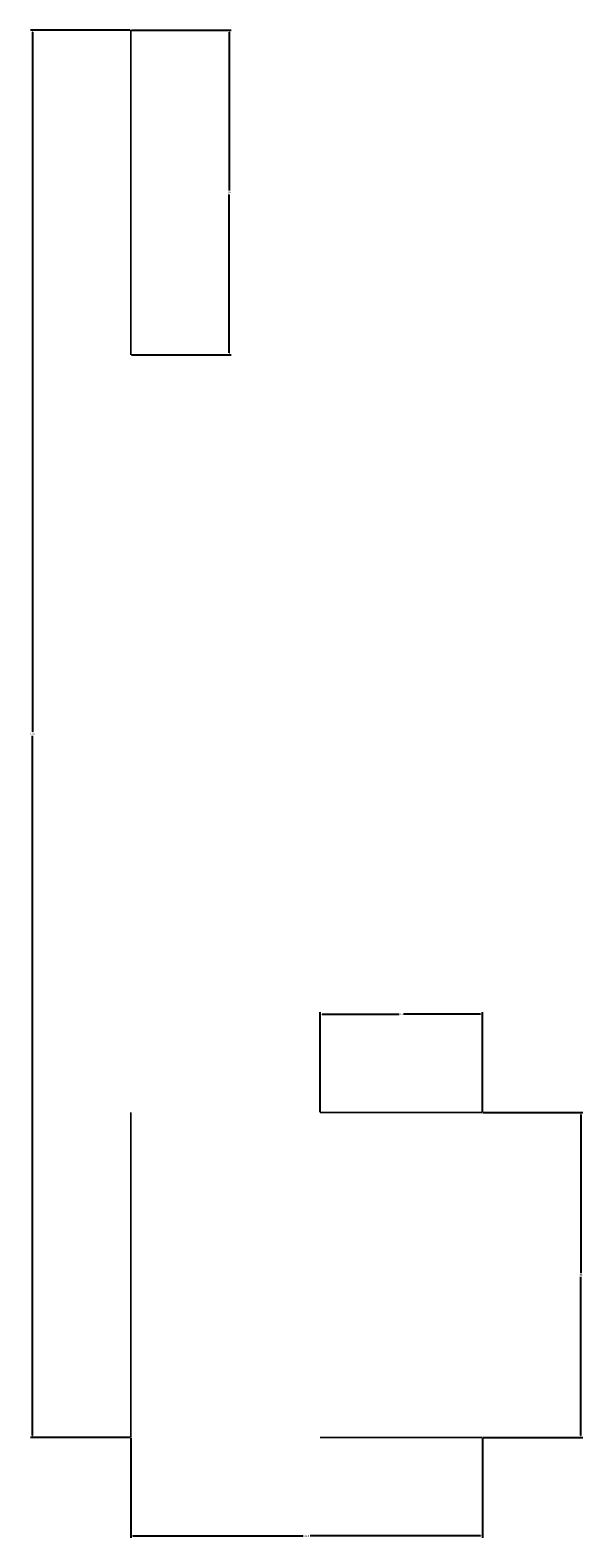
# Model space of a CAD drawing. Units: millimetres. Extents: x -9 to 42, y 320 to 460.
import ezdxf

# ---------------------------------------------------------------- set-up
doc = ezdxf.new("R2010")
doc.units = ezdxf.units.MM
doc.layers.add('M-CONS', color=8, linetype='Continuous', lineweight=13)
doc.layers.add('M-DIMS', color=2, linetype='Continuous', lineweight=18)
doc.styles.get("Standard").update_dxf_attribs({"font": 'arial.ttf'})
doc.dimstyles.get("Standard").update_dxf_attribs({"dimtxt": 0.18, "dimasz": 0.18, "dimexe": 0.18, "dimexo": 0.0625, "dimgap": 0.09, "dimtad": 0, "dimtih": 1, "dimtoh": 1, "dimdec": 4, "dimzin": 0, "dimdsep": 46, "dimtxsty": 'Standard', "dimcen": 0.09, "dimadec": 0, "dimazin": 0, "dimtfac": 1, "dimtdec": 4, "dimtofl": 0, "dimtmove": 0, "dimatfit": 3, "dimfxl": 1, "dimtolj": 1, "dimtzin": 0, "dimarcsym": 0})

# ---------------------------------------------------------------- blocks, each defined once
blk = doc.blocks.new('*D3')
at = {"layer": 'Defpoints', "color": 0, "transparency": 16777216}
for p in [(0, 329.55), (32.5, 329.55), (32.5, 320.45)]:
    blk.add_point(p, dxfattribs=at)
at = {"layer": 'M-DIMS', "color": 0, "lineweight": -2, "transparency": 16777216}
for p, q in [((0, 329.49), (0, 320.27)), ((32.5, 329.49), (32.5, 320.27)), ((0.18, 320.45), (15.93, 320.45)), ((32.32, 320.45), (16.57, 320.45))]:
    blk.add_line(p, q, dxfattribs=at)
at = {"layer": 'M-DIMS', "color": 0, "transparency": 16777216}
for points in [[(0.18, 320.48), (0.18, 320.42), (0, 320.45)], [(32.32, 320.48), (32.32, 320.42), (32.5, 320.45)]]:
    blk.add_solid(points, dxfattribs=at)
at = {"layer": 'M-DIMS', "color": 0, "transparency": 16777216, "insert": (16.25, 320.45), "char_height": 0.18, "attachment_point": 5}
blk.add_mtext('\\A1;32.5', dxfattribs=at)
blk = doc.blocks.new('*D4')
at = {"layer": 'Defpoints', "color": 0, "transparency": 16777216}
for p in [(32.5, 368.65), (17.5, 359.55), (32.5, 359.55)]:
    blk.add_point(p, dxfattribs=at)
at = {"layer": 'M-DIMS', "color": 0, "lineweight": -2, "transparency": 16777216}
for p, q in [((17.5, 359.61), (17.5, 368.83)), ((17.68, 368.65), (24.79, 368.65)), ((32.32, 368.65), (25.21, 368.65)), ((32.5, 359.61), (32.5, 368.83))]:
    blk.add_line(p, q, dxfattribs=at)
at = {"layer": 'M-DIMS', "color": 0, "transparency": 16777216}
for points in [[(17.68, 368.68), (17.68, 368.62), (17.5, 368.65)], [(32.32, 368.68), (32.32, 368.62), (32.5, 368.65)]]:
    blk.add_solid(points, dxfattribs=at)
at = {"layer": 'M-DIMS', "color": 0, "transparency": 16777216, "insert": (25, 368.65), "char_height": 0.18, "attachment_point": 5}
blk.add_mtext('\\A1;15', dxfattribs=at)
blk = doc.blocks.new('*D5')
at = {"layer": 'Defpoints', "color": 0, "transparency": 16777216}
for p in [(-9.1, 459.55), (0, 459.55), (0, 329.55)]:
    blk.add_point(p, dxfattribs=at)
at = {"layer": 'M-DIMS', "color": 0, "lineweight": -2, "transparency": 16777216}
for p, q in [((-0.06, 459.55), (-9.28, 459.55)), ((-9.1, 459.37), (-9.1, 394.73)), ((-9.1, 329.73), (-9.1, 394.37)), ((-0.06, 329.55), (-9.28, 329.55))]:
    blk.add_line(p, q, dxfattribs=at)
at = {"layer": 'M-DIMS', "color": 0, "transparency": 16777216}
for points in [[(-9.13, 459.37), (-9.07, 459.37), (-9.1, 459.55)], [(-9.13, 329.73), (-9.07, 329.73), (-9.1, 329.55)]]:
    blk.add_solid(points, dxfattribs=at)
at = {"layer": 'M-DIMS', "color": 0, "transparency": 16777216, "insert": (-9.1, 394.55), "char_height": 0.18, "attachment_point": 5}
blk.add_mtext('\\A1;130', dxfattribs=at)
blk = doc.blocks.new('*D6')
at = {"layer": 'Defpoints', "color": 0, "transparency": 16777216}
for p in [(0, 459.55), (0, 429.55), (9.1, 429.55)]:
    blk.add_point(p, dxfattribs=at)
at = {"layer": 'M-DIMS', "color": 0, "lineweight": -2, "transparency": 16777216}
for p, q in [((0.06, 459.55), (9.28, 459.55)), ((9.1, 459.37), (9.1, 444.73)), ((9.1, 429.73), (9.1, 444.37)), ((0.06, 429.55), (9.28, 429.55))]:
    blk.add_line(p, q, dxfattribs=at)
at = {"layer": 'M-DIMS', "color": 0, "transparency": 16777216}
for points in [[(9.07, 459.37), (9.13, 459.37), (9.1, 459.55)], [(9.07, 429.73), (9.13, 429.73), (9.1, 429.55)]]:
    blk.add_solid(points, dxfattribs=at)
at = {"layer": 'M-DIMS', "color": 0, "transparency": 16777216, "insert": (9.1, 444.55), "char_height": 0.18, "attachment_point": 5}
blk.add_mtext('\\A1;30', dxfattribs=at)
blk = doc.blocks.new('*D7')
at = {"layer": 'Defpoints', "color": 0, "transparency": 16777216}
for p in [(32.5, 359.55), (41.6, 359.55), (32.5, 329.55)]:
    blk.add_point(p, dxfattribs=at)
at = {"layer": 'M-DIMS', "color": 0, "lineweight": -2, "transparency": 16777216}
for p, q in [((32.56, 359.55), (41.78, 359.55)), ((41.6, 359.37), (41.6, 344.73)), ((41.6, 329.73), (41.6, 344.37)), ((32.56, 329.55), (41.78, 329.55))]:
    blk.add_line(p, q, dxfattribs=at)
at = {"layer": 'M-DIMS', "color": 0, "transparency": 16777216}
for points in [[(41.57, 359.37), (41.63, 359.37), (41.6, 359.55)], [(41.57, 329.73), (41.63, 329.73), (41.6, 329.55)]]:
    blk.add_solid(points, dxfattribs=at)
at = {"layer": 'M-DIMS', "color": 0, "transparency": 16777216, "insert": (41.6, 344.55), "char_height": 0.18, "attachment_point": 5}
blk.add_mtext('\\A1;30', dxfattribs=at)

msp = doc.modelspace()

# ---------------------------------------------------------------- linework, layer by layer
at = {"layer": 'M-CONS', "extrusion": (1, 0, 0)}
msp.add_line((0, 459.55, 200.36), (0, 459.55, 230.36), dxfattribs=at)
for points in [[(459.55, 230.36, 1), (429.55, 230.36), (429.55, 170.36, 1), (459.55, 170.36)], [(454.55, 230.36), (454.55, 170.36, -1), (434.55, 170.36), (434.55, 230.36, -1)], [(359.55, 230.36, 1), (329.55, 230.36), (329.55, 170.36, 1), (359.55, 170.36)], [(354.55, 230.36), (354.55, 170.36, -1), (334.55, 170.36), (334.55, 230.36, -1)]]:
    msp.add_lwpolyline(points, format="xyb", close=True, dxfattribs=at)
at = {"layer": 'M-CONS', "extrusion": (0, -1, 0)}
for centre in [(25, 200.36, -359.55), (25, 200.36, -329.55)]:
    msp.add_circle(centre, 7.5, dxfattribs=at)

# ---------------------------------------------------------------- dimensions: what is measured, and where the dimension line sits
at = {"layer": 'M-DIMS'}
for base, p1, p2, angle, picture, middle in [((-9.1, 459.55), (0, 329.55), (0, 459.55), 90, '*D5', (-9.1, 394.55)), ((9.1, 429.55), (0, 459.55), (0, 429.55), 270, '*D6', (9.1, 444.55)), ((41.6, 359.55), (32.5, 329.55), (32.5, 359.55), 90, '*D7', (41.6, 344.55))]:
    dim = msp.add_linear_dim(base=base, p1=p1, p2=p2, angle=angle, dimstyle='Standard', override={"dimdec": 0, "dimlfac": 1, "dimrnd": 0, "dimzin": 0, "dimdsep": 46, "dimlunit": 2}, dxfattribs=at)
    dim.commit()
    dim.dimension.update_dxf_attribs({"geometry": picture, "text_midpoint": middle})
for base, p1, p2, override, picture, middle in [((32.5, 368.65), (17.5, 359.55), (32.5, 359.55), {"dimdec": 0, "dimlfac": 1, "dimrnd": 0, "dimzin": 0, "dimdsep": 46, "dimlunit": 2}, '*D4', (25, 368.65)), ((32.5, 320.45), (0, 329.55), (32.5, 329.55), {"dimdec": 1, "dimlfac": 1, "dimrnd": 0, "dimzin": 0, "dimdsep": 46, "dimlunit": 2}, '*D3', (16.25, 320.45))]:
    dim = msp.add_linear_dim(base=base, p1=p1, p2=p2, dimstyle='Standard', override=override, dxfattribs=at)
    dim.commit()
    dim.dimension.update_dxf_attribs({"geometry": picture, "text_midpoint": middle})

doc.saveas('drawing.dxf')
